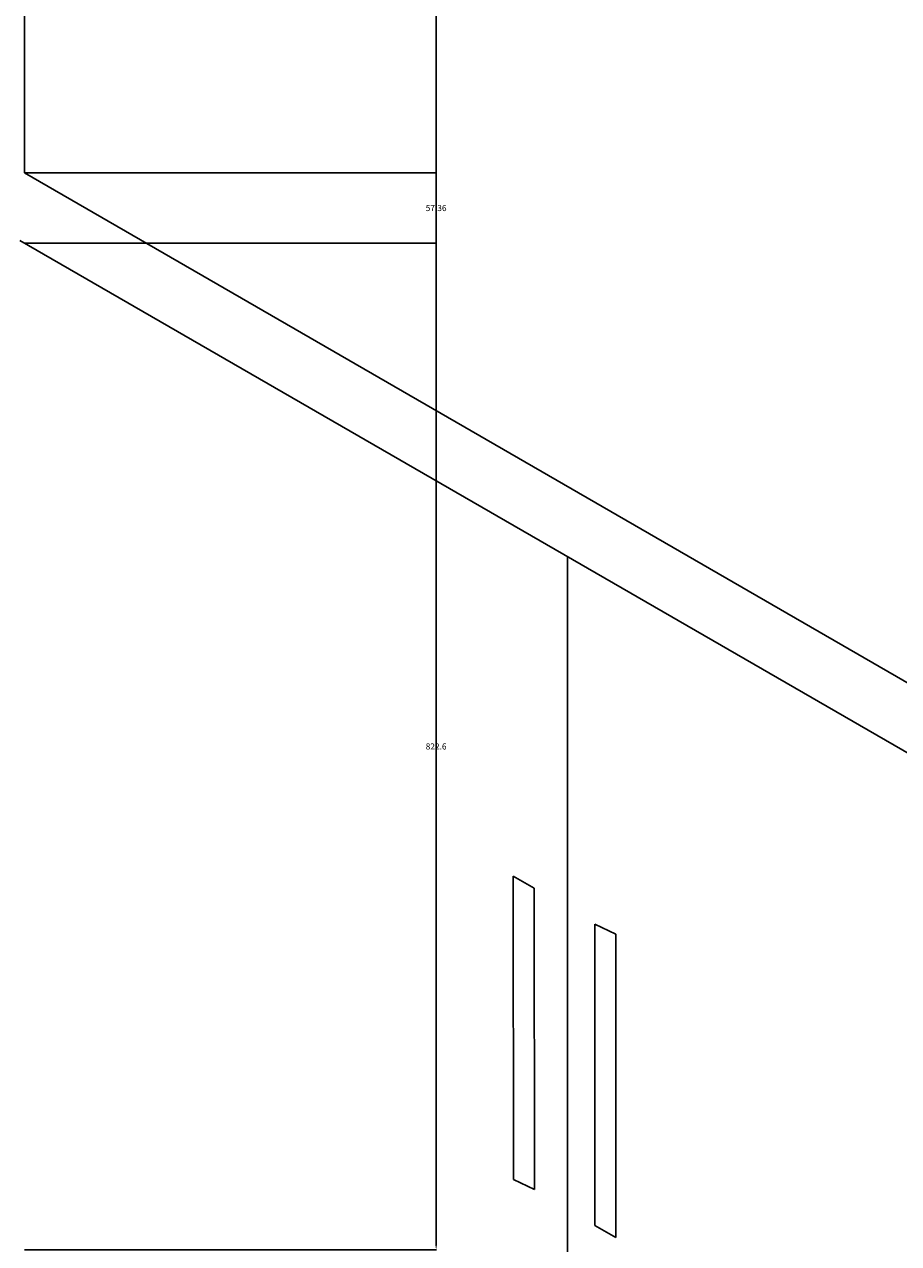
# Model space of a CAD drawing. Units: metres. Extents: x -2391 to 4922, y -635 to 4845.
# Tile 24 of 37: x 551 to 1265, y 2130 to 3127. Entities that reach past the tile are written whole.
import ezdxf

# ---------------------------------------------------------------- set-up
doc = ezdxf.new("R2010")
doc.units = ezdxf.units.M
doc.header["$MEASUREMENT"] = 0
doc.layers.add('A-ANNO-DIMS', color=2, linetype='Continuous', lineweight=18)
doc.layers.add('A-FLOR-FIXT', color=3, linetype='Continuous', lineweight=25)
doc.styles.get("Standard").update_dxf_attribs({"font": 'arial.ttf'})
doc.dimstyles.get("Standard").update_dxf_attribs({"dimtxt": 5, "dimasz": 4, "dimexe": 0.18, "dimexo": 0.0625, "dimgap": 0.09, "dimtad": 0, "dimtih": 1, "dimtoh": 1, "dimdec": 0, "dimzin": 0, "dimdsep": 46, "dimtxsty": 'Standard', "dimcen": 0.09, "dimadec": 0, "dimazin": 0, "dimtfac": 1, "dimtdec": 0, "dimtofl": 0, "dimtmove": 0, "dimatfit": 3, "dimfxl": 1, "dimtolj": 1, "dimtzin": 0, "dimarcsym": 0})

# ---------------------------------------------------------------- blocks, each defined once
blk = doc.blocks.new('HANDLE-DOOR-256')
for p, q in [((0, 256.07), (0, 9.89)), ((0, 256.07), (17.13, 248.01)), ((17.13, 0), (17.13, 248.01)), ((0, 9.89), (17.13, 0))]:
    blk.add_line(p, q)
blk = doc.blocks.new('*D8')
at = {"layer": 'A-ANNO-DIMS', "color": 0, "lineweight": -2, "transparency": 16777216}
for p, q in [((-2047.33, 3005.21), (-2047.33, -631.4)), ((4577.76, 2350.21), (4577.76, -631.4)), ((-2043.33, -631.22), (1257.62, -631.22)), ((4573.76, -631.22), (1272.8, -631.22))]:
    blk.add_line(p, q, dxfattribs=at)
at = {"layer": 'A-ANNO-DIMS', "color": 0, "transparency": 16777216}
for points in [[(-2043.33, -630.56), (-2043.33, -631.89), (-2047.33, -631.22)], [(4573.76, -630.56), (4573.76, -631.89), (4577.76, -631.22)]]:
    blk.add_solid(points, dxfattribs=at)
at = {"layer": 'Defpoints', "color": 0, "transparency": 16777216}
for p in [(-2047.33, 3005.28), (4577.76, 2350.28), (4577.76, -631.22)]:
    blk.add_point(p, dxfattribs=at)
at = {"layer": 'A-ANNO-DIMS', "color": 0, "transparency": 16777216, "insert": (1265.21, -631.22), "char_height": 5, "attachment_point": 5}
blk.add_mtext('\\A1;6625', dxfattribs=at)
blk = doc.blocks.new('*D9')
at = {"layer": 'A-ANNO-DIMS', "color": 0, "lineweight": -2, "transparency": 16777216}
for p, q in [((-2047.33, 3005.34), (-2047.33, 4841.96)), ((-2043.33, 4841.78), (-755.9, 4841.78)), ((546.74, 4841.78), (-740.69, 4841.78)), ((550.74, 4505.34), (550.74, 4841.96))]:
    blk.add_line(p, q, dxfattribs=at)
at = {"layer": 'A-ANNO-DIMS', "color": 0, "transparency": 16777216}
for points in [[(-2043.33, 4842.44), (-2043.33, 4841.11), (-2047.33, 4841.78)], [(546.74, 4842.44), (546.74, 4841.11), (550.74, 4841.78)]]:
    blk.add_solid(points, dxfattribs=at)
at = {"layer": 'Defpoints', "color": 0, "transparency": 16777216}
for p in [(550.74, 4841.78), (550.74, 4505.28), (-2047.33, 3005.28)]:
    blk.add_point(p, dxfattribs=at)
at = {"layer": 'A-ANNO-DIMS', "color": 0, "transparency": 16777216, "insert": (-748.3, 4841.78), "char_height": 5, "attachment_point": 5}
blk.add_mtext('\\A1;2598', dxfattribs=at)
blk = doc.blocks.new('*D10')
at = {"layer": 'A-ANNO-DIMS', "color": 0, "lineweight": -2, "transparency": 16777216}
for p, q in [((550.68, 4505.28), (-2384.01, 4505.28)), ((-2383.83, 4501.28), (-2383.83, 2107.92)), ((-2383.83, -290.72), (-2383.83, 2102.63)), ((-488.55, -294.72), (-2384.01, -294.72))]:
    blk.add_line(p, q, dxfattribs=at)
at = {"layer": 'A-ANNO-DIMS', "color": 0, "transparency": 16777216}
for points in [[(-2384.5, 4501.28), (-2383.17, 4501.28), (-2383.83, 4505.28)], [(-2384.5, -290.72), (-2383.17, -290.72), (-2383.83, -294.72)]]:
    blk.add_solid(points, dxfattribs=at)
at = {"layer": 'Defpoints', "color": 0, "transparency": 16777216}
for p in [(-2383.83, 4505.28), (550.74, 4505.28), (-488.49, -294.72)]:
    blk.add_point(p, dxfattribs=at)
at = {"layer": 'A-ANNO-DIMS', "color": 0, "transparency": 16777216, "insert": (-2383.83, 2105.28), "char_height": 5, "attachment_point": 5}
blk.add_mtext('\\A1;4800', dxfattribs=at)
blk = doc.blocks.new('*D11')
at = {"layer": 'A-ANNO-DIMS', "color": 0, "lineweight": -2, "transparency": 16777216}
for p, q in [((550.8, 4505.28), (887.42, 4505.28)), ((887.24, 4501.28), (887.24, 3317.92)), ((887.24, 2129.28), (887.24, 3312.63)), ((550.8, 2125.28), (887.42, 2125.28))]:
    blk.add_line(p, q, dxfattribs=at)
at = {"layer": 'A-ANNO-DIMS', "color": 0, "transparency": 16777216}
for points in [[(886.58, 4501.28), (887.91, 4501.28), (887.24, 4505.28)], [(886.58, 2129.28), (887.91, 2129.28), (887.24, 2125.28)]]:
    blk.add_solid(points, dxfattribs=at)
at = {"layer": 'Defpoints', "color": 0, "transparency": 16777216}
for p in [(550.74, 4505.28), (550.74, 2125.28), (887.24, 2125.28)]:
    blk.add_point(p, dxfattribs=at)
at = {"layer": 'A-ANNO-DIMS', "color": 0, "transparency": 16777216, "insert": (887.24, 3315.28), "char_height": 5, "attachment_point": 5}
blk.add_mtext('\\A1;2380', dxfattribs=at)
blk = doc.blocks.new('*D17')
at = {"layer": 'A-ANNO-DIMS', "color": 0, "lineweight": -2, "transparency": 16777216}
for p, q in [((550.74, 3005.34), (550.74, 4841.96)), ((554.74, 4841.78), (1014.86, 4841.78)), ((1492.03, 4841.78), (1031.91, 4841.78)), ((1496.03, 2662.52), (1496.03, 4841.96))]:
    blk.add_line(p, q, dxfattribs=at)
at = {"layer": 'A-ANNO-DIMS', "color": 0, "transparency": 16777216}
for points in [[(554.74, 4842.44), (554.74, 4841.11), (550.74, 4841.78)], [(1492.03, 4842.44), (1492.03, 4841.11), (1496.03, 4841.78)]]:
    blk.add_solid(points, dxfattribs=at)
at = {"layer": 'Defpoints', "color": 0, "transparency": 16777216}
for p in [(1496.03, 4841.78), (550.74, 3005.28), (1496.03, 2662.46)]:
    blk.add_point(p, dxfattribs=at)
at = {"layer": 'A-ANNO-DIMS', "color": 0, "transparency": 16777216, "insert": (1023.39, 4841.78), "char_height": 5, "attachment_point": 5}
blk.add_mtext('\\A1;945.3', dxfattribs=at)
blk = doc.blocks.new('*D23')
at = {"layer": 'A-ANNO-DIMS', "color": 0, "lineweight": -2, "transparency": 16777216}
for p, q in [((550.8, 3005.28), (887.42, 3005.28)), ((887.24, 3001.28), (887.24, 2979.24)), ((887.24, 2951.92), (887.24, 2973.95)), ((550.8, 2947.92), (887.42, 2947.92))]:
    blk.add_line(p, q, dxfattribs=at)
at = {"layer": 'A-ANNO-DIMS', "color": 0, "transparency": 16777216}
for points in [[(886.58, 3001.28), (887.91, 3001.28), (887.24, 3005.28)], [(886.58, 2951.92), (887.91, 2951.92), (887.24, 2947.92)]]:
    blk.add_solid(points, dxfattribs=at)
at = {"layer": 'Defpoints', "color": 0, "transparency": 16777216}
for p in [(550.74, 3005.28), (550.74, 2947.92), (887.24, 2947.92)]:
    blk.add_point(p, dxfattribs=at)
at = {"layer": 'A-ANNO-DIMS', "color": 0, "transparency": 16777216, "insert": (887.24, 2976.6), "char_height": 5, "attachment_point": 5}
blk.add_mtext('\\A1;57.36', dxfattribs=at)
blk = doc.blocks.new('*D24')
at = {"layer": 'A-ANNO-DIMS', "color": 0, "lineweight": -2, "transparency": 16777216}
for p, q in [((550.8, 2947.92), (887.42, 2947.92)), ((887.24, 2943.92), (887.24, 2539.24)), ((887.24, 2129.28), (887.24, 2533.96)), ((550.8, 2125.28), (887.42, 2125.28))]:
    blk.add_line(p, q, dxfattribs=at)
at = {"layer": 'A-ANNO-DIMS', "color": 0, "transparency": 16777216}
for points in [[(886.58, 2943.92), (887.91, 2943.92), (887.24, 2947.92)], [(886.58, 2129.28), (887.91, 2129.28), (887.24, 2125.28)]]:
    blk.add_solid(points, dxfattribs=at)
at = {"layer": 'Defpoints', "color": 0, "transparency": 16777216}
for p in [(550.74, 2947.92), (550.74, 2125.28), (887.24, 2125.28)]:
    blk.add_point(p, dxfattribs=at)
at = {"layer": 'A-ANNO-DIMS', "color": 0, "transparency": 16777216, "insert": (887.24, 2536.6), "char_height": 5, "attachment_point": 5}
blk.add_mtext('\\A1;822.6', dxfattribs=at)
blk = doc.blocks.new('*D35')
at = {"layer": 'A-ANNO-DIMS', "color": 0, "lineweight": -2, "transparency": 16777216}
for p, q in [((550.8, 3684.51), (887.42, 3684.51)), ((887.24, 3680.51), (887.24, 3347.54)), ((887.24, 3009.28), (887.24, 3342.25)), ((550.8, 3005.28), (887.42, 3005.28))]:
    blk.add_line(p, q, dxfattribs=at)
at = {"layer": 'A-ANNO-DIMS', "color": 0, "transparency": 16777216}
for points in [[(886.58, 3680.51), (887.91, 3680.51), (887.24, 3684.51)], [(886.58, 3009.28), (887.91, 3009.28), (887.24, 3005.28)]]:
    blk.add_solid(points, dxfattribs=at)
at = {"layer": 'Defpoints', "color": 0, "transparency": 16777216}
for p in [(550.74, 3684.51), (550.74, 3005.28), (887.24, 3005.28)]:
    blk.add_point(p, dxfattribs=at)
at = {"layer": 'A-ANNO-DIMS', "color": 0, "transparency": 16777216, "insert": (887.24, 3344.9), "char_height": 5, "attachment_point": 5}
blk.add_mtext('\\A1;679.2', dxfattribs=at)

msp = doc.modelspace()

# ---------------------------------------------------------------- linework, layer by layer
at = {"layer": 'A-FLOR-FIXT'}
for p, q in [((550.7419, 3005.2763), (3148.8181, 1505.2763)), ((546.8938, 2950.1416), (3148.8181, 1447.9199)), ((994.5103, 2691.71), (994.5103, 1869.0664))]:
    msp.add_line(p, q, dxfattribs=at)

# ---------------------------------------------------------------- block references
at = {"layer": 'A-FLOR-FIXT', "rotation": 180.0273381069543}
msp.add_blockref('HANDLE-DOOR-256', (967.4183, 2430.6881), dxfattribs=at)
at = {"layer": 'A-FLOR-FIXT'}
msp.add_blockref('HANDLE-DOOR-256', (1016.865, 2135.293), dxfattribs=at)

# ---------------------------------------------------------------- dimensions: what is measured, and where the dimension line sits
at = {"layer": 'A-ANNO-DIMS'}
for base, p1, p2, override, picture, middle in [((550.7419, 4841.7763), (-2047.3343, 3005.2763), (550.7419, 4505.2763), {"dimdec": 0, "dimlfac": 1, "dimrnd": 0, "dimzin": 0, "dimdsep": 46, "dimlunit": 2}, '*D9', (-748.2962, 4841.7763)), ((1496.0309, 4841.7763), (550.7419, 3005.2763), (1496.0309, 2662.4566), {"dimdec": 1, "dimlfac": 1, "dimrnd": 0, "dimzin": 0, "dimdsep": 46, "dimlunit": 2}, '*D17', (1023.3864, 4841.7763)), ((4577.76, -631.2237), (-2047.3343, 3005.2763), (4577.76, 2350.2763), {"dimdec": 0, "dimlfac": 1, "dimrnd": 0, "dimzin": 0, "dimdsep": 46, "dimlunit": 2}, '*D8', (1265.2128, -631.2237))]:
    dim = msp.add_linear_dim(base=base, p1=p1, p2=p2, dimstyle='Standard', override=override, dxfattribs=at)
    dim.commit()
    dim.dimension.update_dxf_attribs({"geometry": picture, "text_midpoint": middle})
for base, p1, p2, angle, override, picture, middle in [((-2383.8343, 4505.2763), (-488.4886, -294.7237), (550.7419, 4505.2763), 90, {"dimdec": 0, "dimlfac": 1, "dimrnd": 0, "dimzin": 0, "dimdsep": 46, "dimlunit": 2}, '*D10', (-2383.8343, 2105.2763)), ((887.2419, 2125.2763), (550.7419, 4505.2763), (550.7419, 2125.2763), 270, {"dimdec": 0, "dimlfac": 1, "dimrnd": 0, "dimzin": 0, "dimdsep": 46, "dimlunit": 2}, '*D11', (887.2419, 3315.2763)), ((887.2419, 3005.2763), (550.7419, 3684.5146), (550.7419, 3005.2763), 270, {"dimdec": 1, "dimlfac": 1, "dimrnd": 0, "dimzin": 0, "dimdsep": 46, "dimlunit": 2}, '*D35', (887.2419, 3344.8954)), ((887.2419, 2947.9199), (550.7419, 3005.2763), (550.7419, 2947.9199), 270, {"dimdec": 2, "dimlfac": 1, "dimrnd": 0, "dimzin": 0, "dimdsep": 46, "dimlunit": 2}, '*D23', (887.2419, 2976.5981)), ((887.2419, 2125.2763), (550.7419, 2947.9199), (550.7419, 2125.2763), 270, {"dimdec": 1, "dimlfac": 1, "dimrnd": 0, "dimzin": 0, "dimdsep": 46, "dimlunit": 2}, '*D24', (887.2419, 2536.5981))]:
    dim = msp.add_linear_dim(base=base, p1=p1, p2=p2, angle=angle, dimstyle='Standard', override=override, dxfattribs=at)
    dim.commit()
    dim.dimension.update_dxf_attribs({"geometry": picture, "text_midpoint": middle})

doc.saveas('drawing.dxf')
